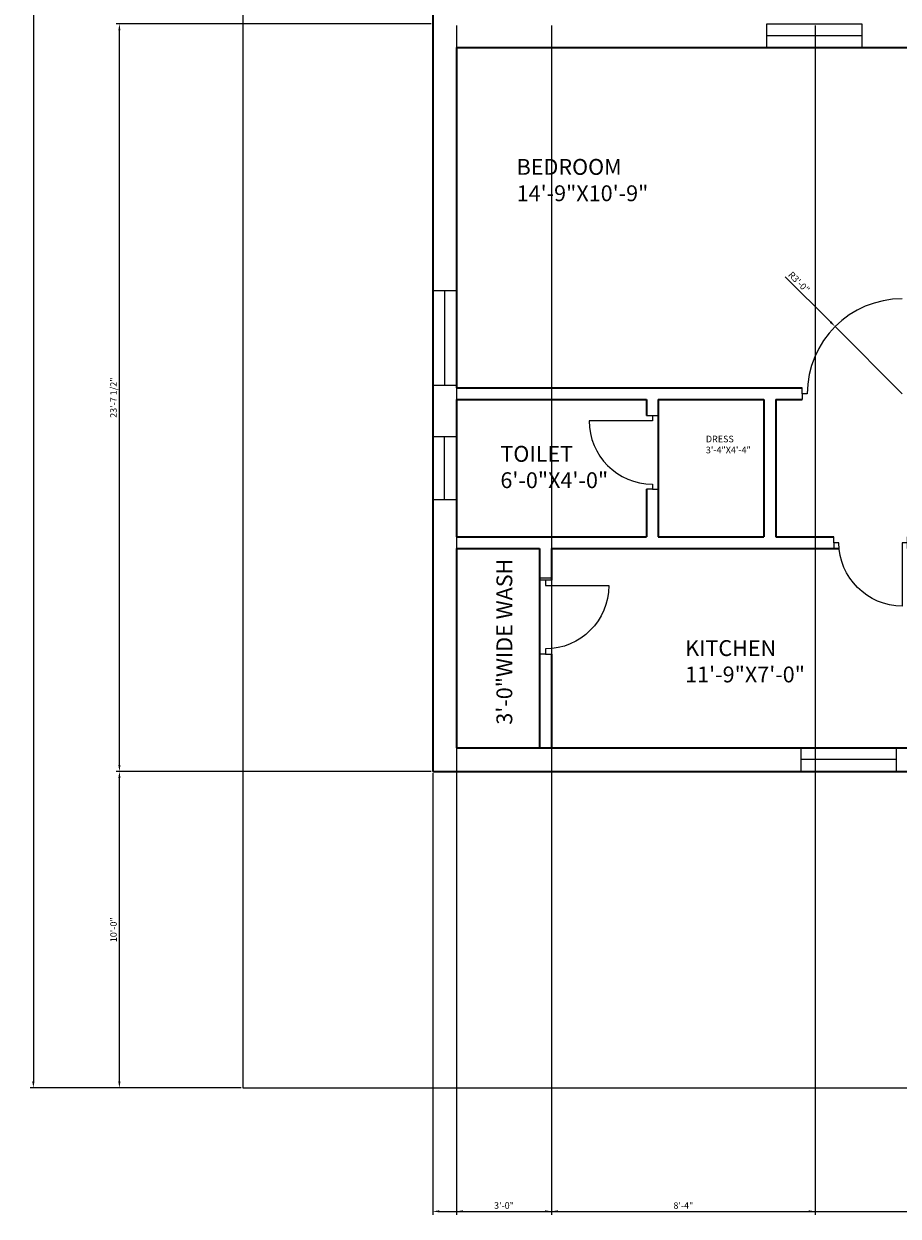
# Model space of a CAD drawing. Units: inches. Extents: x 3257 to 4085, y -12 to 956.
# Tile 1 of 6: x 3257 to 3588, y -12 to 441. Entities that reach past the tile are written whole.
import ezdxf

# ---------------------------------------------------------------- set-up
doc = ezdxf.new("R2010")
doc.units = ezdxf.units.IN
for name, color, linetype, lineweight in [('A-ANNO-DIMS', 2, 'Continuous', 18), ('A-AREA-IDEN', 7, 'Continuous', 18), ('A-DOOR', 3, 'Continuous', 18), ('A-GLAZ', 4, 'Continuous', 18), ('A-WALL', 7, 'Continuous', 35), ('C-PROP', 6, 'Continuous', 25)]:
    doc.layers.add(name, color=color, linetype=linetype, lineweight=lineweight)
doc.styles.get("Standard").update_dxf_attribs({"font": 'arial.ttf'})
doc.dimstyles.new('ISO-25', dxfattribs={"dimtxt": 2.5, "dimasz": 2.5, "dimexe": 1.25, "dimexo": 0.625, "dimtad": 1, "dimdec": 0, "dimlunit": 3, "dimtxsty": 'Standard', "dimcen": 2.5, "dimadec": 0, "dimazin": 0, "dimtfac": 1, "dimtdec": 0, "dimtmove": 0, "dimatfit": 3, "dimfxl": 1, "dimarcsym": 0})

# ---------------------------------------------------------------- blocks, each defined once
blk = doc.blocks.new('*D2')
at = {"layer": 'A-ANNO-DIMS', "color": 0, "lineweight": -2, "transparency": 16777216}
for p, q in [((3339.34, 876), (3259.3, 876)), ((3260.55, 873.5), (3260.55, 39.5)), ((3339.34, 37), (3259.3, 37))]:
    blk.add_line(p, q, dxfattribs=at)
at = {"layer": 'A-ANNO-DIMS', "color": 0, "transparency": 16777216}
for points in [[(3260.13, 873.5), (3260.97, 873.5), (3260.55, 876)], [(3260.13, 39.5), (3260.97, 39.5), (3260.55, 37)]]:
    blk.add_solid(points, dxfattribs=at)
at = {"layer": 'Defpoints', "color": 0, "transparency": 16777216}
for p in [(3339.97, 876), (3260.55, 37), (3339.97, 37)]:
    blk.add_point(p, dxfattribs=at)
at = {"layer": 'A-ANNO-DIMS', "color": 0, "transparency": 16777216, "insert": (3258.65, 456.5), "char_height": 2.5, "attachment_point": 5, "rotation": 90}
blk.add_mtext('71\'-0"', dxfattribs=at)
blk = doc.blocks.new('DOOR-SGL-24IN')
for p, q in [((2.25, 28), (0, 28)), ((2.25, 26), (2.25, 28)), ((2.25, 28), (4.5, 28)), ((2.25, 0), (2.25, 2)), ((2.25, 2), (26.25, 2)), ((4.5, 0), (0, 0))]:
    blk.add_line(p, q)
blk.add_arc((2.25, 2), 24, 0, 90)
blk = doc.blocks.new('WIN-36IN')
for p, q in [((0, 9), (36, 9)), ((0, 0), (0, 9)), ((36, 9), (36, 0)), ((0, 4.5), (36, 4.5)), ((36, 0), (0, 0))]:
    blk.add_line(p, q)
blk = doc.blocks.new('WIN-24IN')
for p, q in [((0, 9), (24, 9)), ((0, 0), (0, 9)), ((24, 9), (24, 0)), ((0, 4.5), (24, 4.5)), ((24, 0), (0, 0))]:
    blk.add_line(p, q)
blk = doc.blocks.new('*D18')
at = {"layer": 'A-ANNO-DIMS', "color": 0, "lineweight": -2, "transparency": 16777216}
for p, q in [((3411.97, 156.38), (3411.97, -11.05)), ((3964.47, 156.38), (3964.47, -11.05)), ((3414.47, -9.8), (3961.97, -9.8))]:
    blk.add_line(p, q, dxfattribs=at)
at = {"layer": 'A-ANNO-DIMS', "color": 0, "transparency": 16777216}
for points in [[(3414.47, -9.38), (3414.47, -10.21), (3411.97, -9.8)], [(3961.97, -9.38), (3961.97, -10.21), (3964.47, -9.8)]]:
    blk.add_solid(points, dxfattribs=at)
at = {"layer": 'Defpoints', "color": 0, "transparency": 16777216}
for p in [(3411.97, 157), (3964.47, 157), (3964.47, -9.8)]:
    blk.add_point(p, dxfattribs=at)
at = {"layer": 'A-ANNO-DIMS', "color": 0, "transparency": 16777216, "insert": (3688.22, -7.88), "char_height": 2.5, "attachment_point": 5}
blk.add_mtext('46\'-0 1/2"', dxfattribs=at)
blk = doc.blocks.new('*D21')
at = {"layer": 'A-ANNO-DIMS', "color": 0, "lineweight": -2, "transparency": 16777216}
for p, q in [((3411.34, 157), (3291.92, 157)), ((3293.17, 39.5), (3293.17, 154.5)), ((3339.34, 37), (3291.92, 37))]:
    blk.add_line(p, q, dxfattribs=at)
at = {"layer": 'A-ANNO-DIMS', "color": 0, "transparency": 16777216}
for points in [[(3292.75, 154.5), (3293.58, 154.5), (3293.17, 157)], [(3292.75, 39.5), (3293.58, 39.5), (3293.17, 37)]]:
    blk.add_solid(points, dxfattribs=at)
at = {"layer": 'Defpoints', "color": 0, "transparency": 16777216}
for p in [(3293.17, 157), (3411.97, 157), (3339.97, 37)]:
    blk.add_point(p, dxfattribs=at)
at = {"layer": 'A-ANNO-DIMS', "color": 0, "transparency": 16777216, "insert": (3291.27, 97), "char_height": 2.5, "attachment_point": 5, "rotation": 90}
blk.add_mtext('10\'-0"', dxfattribs=at)
blk = doc.blocks.new('*D22')
at = {"layer": 'A-ANNO-DIMS', "color": 0, "lineweight": -2, "transparency": 16777216}
for p, q in [((3411.34, 440.5), (3291.92, 440.5)), ((3293.17, 159.5), (3293.17, 438)), ((3411.34, 157), (3291.92, 157))]:
    blk.add_line(p, q, dxfattribs=at)
at = {"layer": 'A-ANNO-DIMS', "color": 0, "transparency": 16777216}
for points in [[(3292.75, 438), (3293.58, 438), (3293.17, 440.5)], [(3292.75, 159.5), (3293.58, 159.5), (3293.17, 157)]]:
    blk.add_solid(points, dxfattribs=at)
at = {"layer": 'Defpoints', "color": 0, "transparency": 16777216}
for p in [(3293.17, 440.5), (3411.97, 440.5), (3411.97, 157)]:
    blk.add_point(p, dxfattribs=at)
at = {"layer": 'A-ANNO-DIMS', "color": 0, "transparency": 16777216, "insert": (3291.25, 298.75), "char_height": 2.5, "attachment_point": 5, "rotation": 90}
blk.add_mtext('23\'-7 1/2"', dxfattribs=at)
blk = doc.blocks.new('*D23')
at = {"layer": 'A-ANNO-DIMS', "color": 0, "lineweight": -2, "transparency": 16777216}
for p, q in [((3420.97, 439.88), (3420.97, -11.05)), ((3456.97, 439.88), (3456.97, -11.05)), ((3423.47, -9.8), (3454.47, -9.8))]:
    blk.add_line(p, q, dxfattribs=at)
at = {"layer": 'A-ANNO-DIMS', "color": 0, "transparency": 16777216}
for points in [[(3423.47, -9.38), (3423.47, -10.21), (3420.97, -9.8)], [(3454.47, -9.38), (3454.47, -10.21), (3456.97, -9.8)]]:
    blk.add_solid(points, dxfattribs=at)
at = {"layer": 'Defpoints', "color": 0, "transparency": 16777216}
for p in [(3420.97, 440.5), (3456.97, 440.5), (3456.97, -9.8)]:
    blk.add_point(p, dxfattribs=at)
at = {"layer": 'A-ANNO-DIMS', "color": 0, "transparency": 16777216, "insert": (3438.97, -7.89), "char_height": 2.5, "attachment_point": 5}
blk.add_mtext('3\'-0"', dxfattribs=at)
blk = doc.blocks.new('*D24')
at = {"layer": 'A-ANNO-DIMS', "color": 0, "lineweight": -2, "transparency": 16777216}
for p, q in [((3456.97, 439.88), (3456.97, -11.05)), ((3556.97, 439.88), (3556.97, -11.05)), ((3459.47, -9.8), (3554.47, -9.8))]:
    blk.add_line(p, q, dxfattribs=at)
at = {"layer": 'A-ANNO-DIMS', "color": 0, "transparency": 16777216}
for points in [[(3459.47, -9.38), (3459.47, -10.21), (3456.97, -9.8)], [(3554.47, -9.38), (3554.47, -10.21), (3556.97, -9.8)]]:
    blk.add_solid(points, dxfattribs=at)
at = {"layer": 'Defpoints', "color": 0, "transparency": 16777216}
for p in [(3456.97, 440.5), (3556.97, 440.5), (3556.97, -9.8)]:
    blk.add_point(p, dxfattribs=at)
at = {"layer": 'A-ANNO-DIMS', "color": 0, "transparency": 16777216, "insert": (3506.97, -7.9), "char_height": 2.5, "attachment_point": 5}
blk.add_mtext('8\'-4"', dxfattribs=at)
blk = doc.blocks.new('*D28')
at = {"layer": 'A-ANNO-DIMS', "color": 0, "lineweight": -2, "transparency": 16777216}
for p, q in [((3545.6, 344.62), (3562.74, 327.48)), ((3589.97, 300.25), (3564.51, 325.71))]:
    blk.add_line(p, q, dxfattribs=at)
at = {"layer": 'A-ANNO-DIMS', "color": 0, "transparency": 16777216}
blk.add_solid([(3563.04, 327.77), (3562.45, 327.18), (3564.51, 325.71)], dxfattribs=at)
at = {"layer": 'Defpoints', "color": 0, "transparency": 16777216}
for p in [(3564.51, 325.71), (3589.97, 300.25)]:
    blk.add_point(p, dxfattribs=at)
at = {"layer": 'A-ANNO-DIMS', "color": 0, "transparency": 16777216, "insert": (3550.58, 342.33), "char_height": 2.5, "attachment_point": 5, "rotation": 314.9996}
blk.add_mtext('R3\'-0"', dxfattribs=at)

msp = doc.modelspace()

# ---------------------------------------------------------------- linework, layer by layer
at = {"layer": 'A-DOOR'}
for p, q in [((3551.97, 300.25), (3551.97, 302.5)), ((3553.97, 300.25), (3551.97, 300.25)), ((3551.97, 300.25), (3551.97, 298)), ((3452.47, 230.5), (3456.97, 230.5))]:
    msp.add_line(p, q, dxfattribs=at)
msp.add_arc((3589.97, 300.25), 36, 90, 180, dxfattribs=at)
at = {"layer": 'A-WALL'}
for p, q in [((3411.97, 745), (3411.97, 157)), ((3420.97, 431.5), (3826.97, 431.5)), ((3420.97, 431.5), (3420.97, 302.5)), ((3420.97, 302.5), (3551.97, 302.5)), ((3420.97, 298), (3492.97, 298)), ((3420.97, 298), (3420.97, 246)), ((3492.97, 298), (3492.97, 292)), ((3492.97, 294.07), (3492.97, 294.07)), ((3497.47, 298), (3497.47, 246)), ((3497.47, 298), (3537.47, 298)), ((3497.47, 294.68), (3497.47, 294.68)), ((3537.47, 298), (3537.47, 246)), ((3541.97, 298), (3541.97, 246)), ((3541.97, 298), (3551.97, 298)), ((3492.97, 264), (3492.97, 246)), ((3420.97, 246), (3452.47, 246)), ((3452.47, 246), (3456.97, 246)), ((3456.97, 246), (3492.97, 246)), ((3497.47, 246), (3537.47, 246)), ((3541.97, 246), (3563.97, 246)), ((3420.97, 241.5), (3452.47, 241.5)), ((3420.97, 241.5), (3420.97, 166)), ((3452.47, 241.5), (3452.47, 166)), ((3456.97, 241.5), (3456.97, 229.5)), ((3456.97, 241.5), (3566.07, 241.5)), ((3456.97, 201.5), (3456.97, 166)), ((3420.97, 166), (3955.47, 166)), ((3411.97, 157), (3964.47, 157))]:
    msp.add_line(p, q, dxfattribs=at)
at = {"layer": 'C-PROP'}
for p, q in [((3339.97, 745), (3339.97, 37)), ((3339.97, 37), (3411.97, 37)), ((3411.97, 37), (3964.47, 37))]:
    msp.add_line(p, q, dxfattribs=at)

# ---------------------------------------------------------------- block references
at = {"layer": 'A-DOOR', "rotation": 180}
msp.add_blockref('DOOR-SGL-24IN', (3497.47, 292), dxfattribs=at)
at = {"layer": 'A-DOOR', "extrusion": (0, 0, -1), "zscale": -1}
for p, rotation in [((-3591.97, 246), 269.9999999999996), ((-3452.47, 229.5), 179.9997874155053)]:
    msp.add_blockref('DOOR-SGL-24IN', p, dxfattribs=dict(at, rotation=rotation))
at = {"layer": 'A-GLAZ'}
for name, p, rotation in [('WIN-36IN', (3574.64, 440.5), 180), ('WIN-36IN', (3411.97, 339.37), 270.0000000000014), ('WIN-24IN', (3420.97, 260), 90.0000000000012), ('WIN-36IN', (3587.68, 166), 180)]:
    msp.add_blockref(name, p, dxfattribs=dict(at, rotation=rotation))

# ---------------------------------------------------------------- texts
at = {"layer": 'A-AREA-IDEN', "attachment_point": 1}
for s, insert, char_height in [('BEDROOM\\P14\'-9"X10\'-9" ', (3443.76, 389.26), 6), ('TOILET\\P6\'-0"X4\'-0"', (3437.61, 280.45), 6), ('DRESS\\P3\'-4"X4\'-4"', (3515.51, 284.33), 2.5), ('KITCHEN\\P11\'-9"X7\'-0" ', (3507.66, 206.8), 6)]:
    msp.add_mtext(s, dxfattribs=dict(at, insert=insert, char_height=char_height))
at = {"layer": 'A-AREA-IDEN', "insert": (3436.11, 174.74), "char_height": 6, "attachment_point": 1, "rotation": 90}
msp.add_mtext('3\'-0"WIDE WASH', dxfattribs=at)

# ---------------------------------------------------------------- dimensions: what is measured, and where the dimension line sits
at = {"layer": 'A-ANNO-DIMS'}
dim = msp.add_linear_dim(base=(3260.55, 37), p1=(3339.97, 876), p2=(3339.97, 37), angle=90, text='71\'-0"', dimstyle='ISO-25', override={"dimclrd": 0, "dimclre": 0, "dimclrt": 0}, dxfattribs=at)
dim.commit()
dim.dimension.update_dxf_attribs({"geometry": '*D2', "text_midpoint": (3258.65, 456.5)})
for base, p1, p2, picture, middle in [((3293.17, 440.5), (3411.97, 157), (3411.97, 440.5), '*D22', (3291.25, 298.75)), ((3293.17, 157), (3339.97, 37), (3411.97, 157), '*D21', (3291.27, 97))]:
    dim = msp.add_linear_dim(base=base, p1=p1, p2=p2, angle=90, dimstyle='ISO-25', override={"dimdec": 1, "dimlfac": 1, "dimrnd": 0, "dimzin": 1, "dimdsep": 46, "dimlunit": 4, "dimfrac": 2}, dxfattribs=at)
    dim.commit()
    dim.dimension.update_dxf_attribs({"geometry": picture, "text_midpoint": middle})
for base, p1, p2, picture, middle in [((3456.97, -9.8), (3420.97, 440.5), (3456.97, 440.5), '*D23', (3438.97, -7.89)), ((3556.97, -9.8), (3456.97, 440.5), (3556.97, 440.5), '*D24', (3506.97, -7.9)), ((3964.47, -9.8), (3411.97, 157), (3964.47, 157), '*D18', (3688.22, -7.88))]:
    dim = msp.add_linear_dim(base=base, p1=p1, p2=p2, dimstyle='ISO-25', override={"dimdec": 1, "dimlfac": 1, "dimrnd": 0, "dimzin": 1, "dimdsep": 46, "dimlunit": 4, "dimfrac": 2}, dxfattribs=at)
    dim.commit()
    dim.dimension.update_dxf_attribs({"geometry": picture, "text_midpoint": middle})
dim = msp.add_radius_dim(center=(3589.97, 300.25), mpoint=(3564.51, 325.71), dimstyle='ISO-25', override={"dimdec": 1, "dimlfac": 1, "dimrnd": 0, "dimzin": 1, "dimdsep": 46, "dimlunit": 4, "dimfrac": 2}, dxfattribs=at)
dim.commit()
dim.dimension.update_dxf_attribs({"geometry": '*D28', "text_midpoint": (3549.24, 340.98), "dimtype": 164})

doc.saveas('drawing.dxf')
